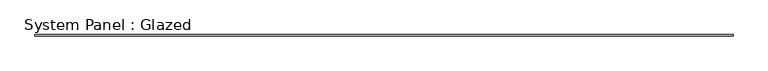
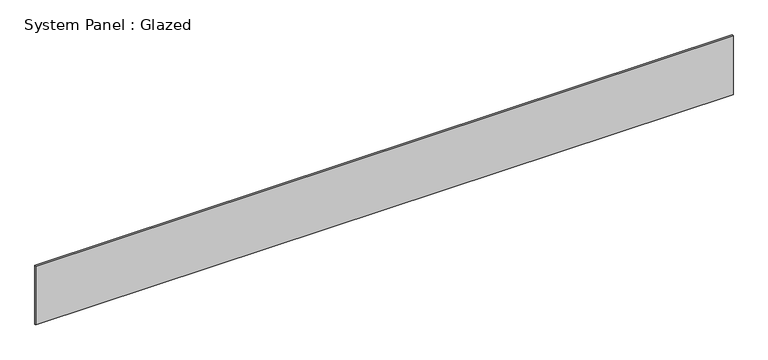
"""IFC4 building model written with IfcOpenShell, lengths in millimetres: plate geometry, System Panel : Glazed."""

from ifc_helpers import new_model, si_unit, origin, origin_with_axes, place, context, project, spatial, polyline, outline, extrude, source, transform, mapped, element, save


def system_panel_glazed_547c043f(model_context):
    return source(origin(), model_context, "Body", "SweptSolid", [
        extrude(outline(polyline([(6477.0, 19.05), (-6477.0, 19.05), (-6477.0, 44.45), (6477.0, 44.45), (6477.0, 19.05)])), origin_with_axes(), (0.0, 0.0, 1.0), 1155.7),
    ])


if __name__ == "__main__":
    model = new_model("IFC4")
    model_context = context("Model", 3, world=origin())
    ifc_project = project(units=[si_unit("LENGTHUNIT", "METRE", prefix="MILLI")], contexts=[model_context])
    site = spatial("IfcSite", under=ifc_project)
    building = spatial("IfcBuilding", under=site)
    placement = place(None, origin())
    system_panel_glazed_shape = system_panel_glazed_547c043f(model_context)
    element("IfcPlate", 1, ObjectType="System Panel : Glazed", at=placement, inside=building, context=model_context, shape_type="MappedRepresentation", body=[
        mapped(system_panel_glazed_shape, transform((0.0, 0.0, 0.0), x_axis=(1.0, 0.0, 0.0), y_axis=(0.0, 1.0, 0.0), z_axis=(0.0, 0.0, 1.0))),
    ])
    save(model, "model.ifc")

# Revit data of these elements
# Type "System Panel : Glazed"
#   Construction Type Id = "GSP4R"
#   Analytic Construction = "1/8 in Pilkington single glazing"
#   Visual Light Transmittance = 0.9
#   Solar Heat Gain Coefficient = 0.86
#   Heat Transfer Coefficient (U) = 1.18115 BTU/(h·ft²·°F)
# Element 1 (IfcPlate, "System Panel : Glazed")
#   Materials on its faces: "Glass"
# Materials
#   "Glass": class "Glass", colour RGB 0 128 192, transparency 0.75, Description = "Soda Lime Glass", Cost = 0
